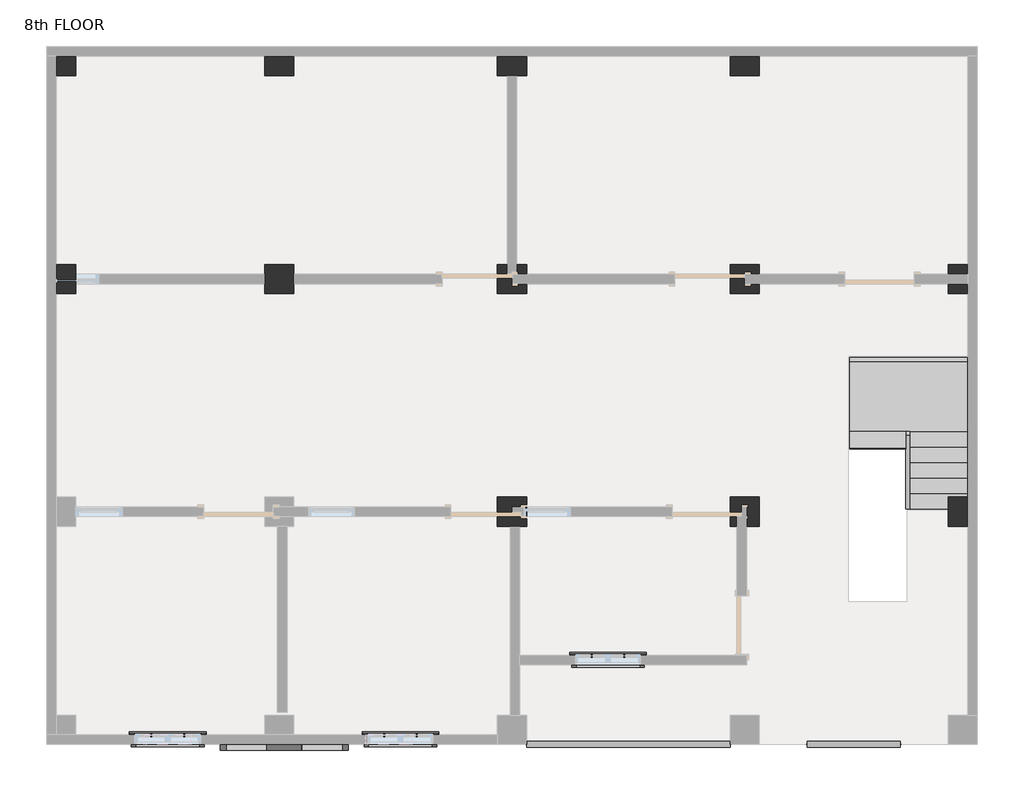
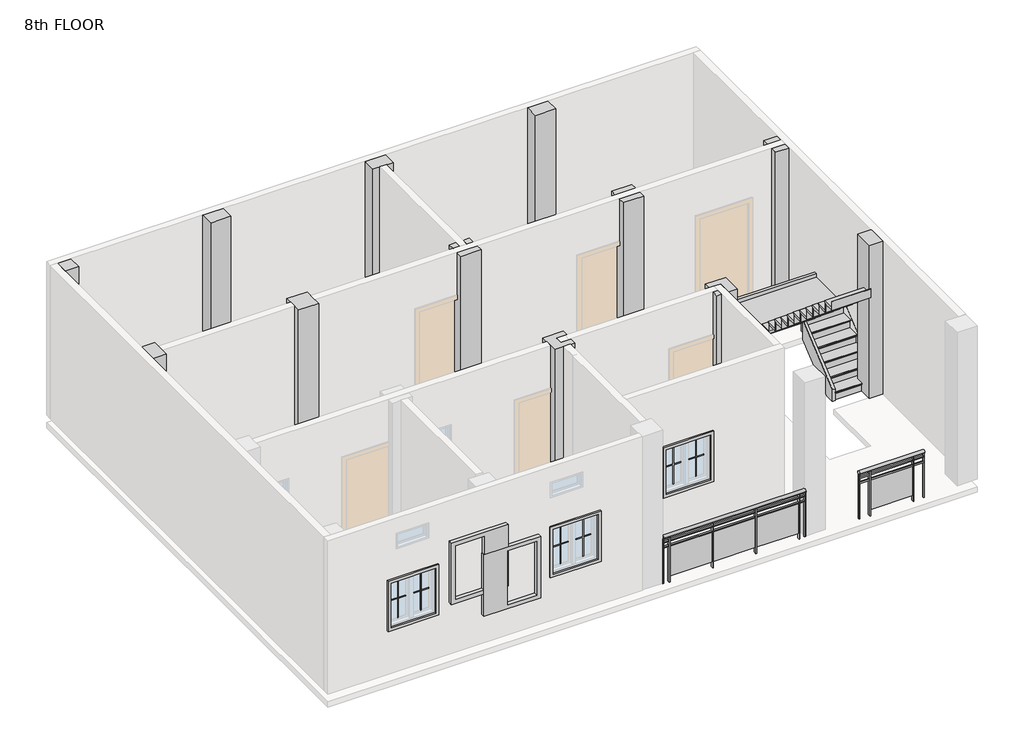
# One storey, part 2 of 2: 12 columns, 12 proxies, 4 members, 2 railings, 1 damper, 1 stair flight.
"""IFC4 building model written with IfcOpenShell, lengths in millimetres."""

from ifc_helpers import new_model, si_unit, point, frame, origin, place, context, project, spatial, polyline, ellipse_curve, trimmed, outline, extrude, faceted_brep, transform, mapped, element, save
from ifc_brep_helpers import plane_surface, extruded_surface, advanced_brep
from components import muntin_pattern_2x2_muntin_pattern_2x2_b3fe6957, muntin_pattern_2x2_muntin_pattern_2x2_3e0ecaf2, trim_window_exterior_flat_with_sill_41619996, trim_window_interior_flat_picture_frame_51c85655, duct_accessories_5_duct_accessories_1_bcda36b2, stair_flight_07a640bc

model = new_model("IFC4")

# Units and contexts
model_context = context("Model", 3, world=origin())
ifc_project = project(units=[si_unit("LENGTHUNIT", "METRE", prefix="MILLI")], contexts=[model_context])

# Site, building, storey
site = spatial("IfcSite", under=ifc_project)
building = spatial("IfcBuilding", under=site)
storey = spatial("IfcBuildingStorey", under=building, Name="8th FLOOR", Elevation=24231.6)

# Proxies
placement = place(None, origin())
muntin_pattern_2x2_muntin_pattern_2x2_shape = muntin_pattern_2x2_muntin_pattern_2x2_b3fe6957(model_context)
element("IfcBuildingElementProxy", 1, Name="Muntin Pattern_2x2 : Muntin Pattern_2x2", ObjectType="Muntin Pattern_2x2 : Muntin Pattern_2x2", at=placement, inside=storey, context=model_context, shape_type="MappedRepresentation", body=[
    mapped(muntin_pattern_2x2_muntin_pattern_2x2_shape, transform((-14441.409625, -253.8184478, 25215.85), x_axis=(1.0, 0.0, 0.0), y_axis=(0.0, 1.0, 0.0), z_axis=(0.0, 0.0, 1.0))),
])
element("IfcBuildingElementProxy", 2, Name="Muntin Pattern_2x2 : Muntin Pattern_2x2", ObjectType="Muntin Pattern_2x2 : Muntin Pattern_2x2", at=placement, inside=storey, context=model_context, shape_type="MappedRepresentation", body=[
    mapped(muntin_pattern_2x2_muntin_pattern_2x2_shape, transform((-11393.409625, -253.8184478, 25215.85), x_axis=(1.0, 0.0, 0.0), y_axis=(0.0, 1.0, 0.0), z_axis=(0.0, 0.0, 1.0))),
])
element("IfcBuildingElementProxy", 3, Name="Muntin Pattern_2x2 : Muntin Pattern_2x2", ObjectType="Muntin Pattern_2x2 : Muntin Pattern_2x2", at=placement, inside=storey, context=model_context, shape_type="MappedRepresentation", body=[
    mapped(muntin_pattern_2x2_muntin_pattern_2x2_shape, transform((-8675.609625, 787.5815522, 25215.85), x_axis=(1.0, 0.0, 0.0), y_axis=(0.0, 1.0, 0.0), z_axis=(0.0, 0.0, 1.0))),
])
muntin_pattern_2x2_muntin_pattern_2x2_2_shape = muntin_pattern_2x2_muntin_pattern_2x2_3e0ecaf2(model_context)
element("IfcBuildingElementProxy", 4, Name="Muntin Pattern_2x2 : Muntin Pattern_2x2", ObjectType="Muntin Pattern_2x2 : Muntin Pattern_2x2", at=placement, inside=storey, context=model_context, shape_type="MappedRepresentation", body=[
    mapped(muntin_pattern_2x2_muntin_pattern_2x2_2_shape, transform((-14012.784625, -253.8184478, 25215.85), x_axis=(-1.0, 0.0, 0.0), y_axis=(0.0, -1.0, 0.0), z_axis=(0.0, 0.0, 1.0))),
])
element("IfcBuildingElementProxy", 5, Name="Muntin Pattern_2x2 : Muntin Pattern_2x2", ObjectType="Muntin Pattern_2x2 : Muntin Pattern_2x2", at=placement, inside=storey, context=model_context, shape_type="MappedRepresentation", body=[
    mapped(muntin_pattern_2x2_muntin_pattern_2x2_2_shape, transform((-10964.784625, -253.8184478, 25215.85), x_axis=(-1.0, 0.0, 0.0), y_axis=(0.0, -1.0, 0.0), z_axis=(0.0, 0.0, 1.0))),
])
element("IfcBuildingElementProxy", 6, Name="Muntin Pattern_2x2 : Muntin Pattern_2x2", ObjectType="Muntin Pattern_2x2 : Muntin Pattern_2x2", at=placement, inside=storey, context=model_context, shape_type="MappedRepresentation", body=[
    mapped(muntin_pattern_2x2_muntin_pattern_2x2_2_shape, transform((-8246.984625, 787.5815522, 25215.85), x_axis=(-1.0, 0.0, 0.0), y_axis=(0.0, -1.0, 0.0), z_axis=(0.0, 0.0, 1.0))),
])
trim_window_exterior_flat_with_sill_shape = trim_window_exterior_flat_with_sill_41619996(model_context)
element("IfcBuildingElementProxy", 7, Name="Trim-Window-Exterior-Flat : with Sill", ObjectType="Trim-Window-Exterior-Flat : with Sill", at=placement, inside=storey, context=model_context, shape_type="MappedRepresentation", body=[
    mapped(trim_window_exterior_flat_with_sill_shape, transform((-14227.097125, -244.2934478, 26060.4), x_axis=(-1.0, 0.0, 0.0), y_axis=(0.0, 0.0, 1.0), z_axis=(0.0, 1.0, 0.0))),
])
element("IfcBuildingElementProxy", 8, Name="Trim-Window-Exterior-Flat : with Sill", ObjectType="Trim-Window-Exterior-Flat : with Sill", at=placement, inside=storey, context=model_context, shape_type="MappedRepresentation", body=[
    mapped(trim_window_exterior_flat_with_sill_shape, transform((-11179.097125, -244.2934478, 26060.4), x_axis=(-1.0, 0.0, 0.0), y_axis=(0.0, 0.0, 1.0), z_axis=(0.0, 1.0, 0.0))),
])
element("IfcBuildingElementProxy", 9, Name="Trim-Window-Exterior-Flat : with Sill", ObjectType="Trim-Window-Exterior-Flat : with Sill", at=placement, inside=storey, context=model_context, shape_type="MappedRepresentation", body=[
    mapped(trim_window_exterior_flat_with_sill_shape, transform((-8461.297125, 797.1065522, 26060.4), x_axis=(-1.0, 0.0, 0.0), y_axis=(0.0, 0.0, 1.0), z_axis=(0.0, 1.0, 0.0))),
])
trim_window_interior_flat_picture_frame_shape = trim_window_interior_flat_picture_frame_51c85655(model_context)
element("IfcBuildingElementProxy", 10, Name="Trim-Window-Interior-Flat : Picture Frame", ObjectType="Trim-Window-Interior-Flat : Picture Frame", at=placement, inside=storey, context=model_context, shape_type="MappedRepresentation", body=[
    mapped(trim_window_interior_flat_picture_frame_shape, transform((-14227.097125, -371.2934478, 26060.4), x_axis=(1.0, 0.0, 0.0), y_axis=(0.0, 0.0, 1.0), z_axis=(0.0, -1.0, 0.0))),
])
element("IfcBuildingElementProxy", 11, Name="Trim-Window-Interior-Flat : Picture Frame", ObjectType="Trim-Window-Interior-Flat : Picture Frame", at=placement, inside=storey, context=model_context, shape_type="MappedRepresentation", body=[
    mapped(trim_window_interior_flat_picture_frame_shape, transform((-11179.097125, -371.2934478, 26060.4), x_axis=(1.0, 0.0, 0.0), y_axis=(0.0, 0.0, 1.0), z_axis=(0.0, -1.0, 0.0))),
])
element("IfcBuildingElementProxy", 12, Name="Trim-Window-Interior-Flat : Picture Frame", ObjectType="Trim-Window-Interior-Flat : Picture Frame", at=placement, inside=storey, context=model_context, shape_type="MappedRepresentation", body=[
    mapped(trim_window_interior_flat_picture_frame_shape, transform((-8461.297125, 670.1065522, 26060.4), x_axis=(1.0, 0.0, 0.0), y_axis=(0.0, 0.0, 1.0), z_axis=(0.0, -1.0, 0.0))),
])

# Columns
element("IfcColumn", 13, ObjectType="column family : column family", at=placement, inside=storey, context=model_context, shape_type="SweptSolid", body=[
    extrude(outline(polyline([(-15433.597125, 8645.7065522), (-15433.597125, 8391.7065522), (-15687.597125, 8391.7065522), (-15687.597125, 8645.7065522), (-15433.597125, 8645.7065522)])), frame((0.0, 0.0, 24236.6), z_axis=(0.0, 0.0, 1.0), x_axis=(1.0, 0.0, 0.0)), (0.0, 0.0, 1.0), 3038.0),
])
element("IfcColumn", 14, ObjectType="column family : column family", at=placement, inside=storey, context=model_context, shape_type="SweptSolid", body=[
    extrude(outline(polyline([(-12576.097125, 5915.2065522), (-12576.097125, 5534.2065522), (-12957.097125, 5534.2065522), (-12957.097125, 5915.2065522), (-12576.097125, 5915.2065522)])), frame((0.0, 0.0, 24236.6), z_axis=(0.0, 0.0, 1.0), x_axis=(1.0, 0.0, 0.0)), (0.0, 0.0, 1.0), 3038.0),
])
element("IfcColumn", 15, ObjectType="column family : column family", at=placement, inside=storey, context=model_context, shape_type="Brep", body=[
    faceted_brep([(-9655.097125, 5915.2065522, 24236.6), (-9528.097125, 5915.2065522, 24236.6), (-9528.097125, 5788.2065522, 24236.6), (-9655.097125, 5788.2065522, 24236.6), (-9528.097125, 5915.2065522, 27274.6), (-9655.097125, 5915.2065522, 27274.6), (-9655.097125, 5788.2065522, 27274.6), (-9528.097125, 5788.2065522, 27274.6)], [[[0, 1, 2, 3]], [[4, 5, 6, 7]], [[0, 3, 6, 5]], [[4, 1, 0, 5]], [[3, 2, 7, 6]], [[1, 4, 7, 2]]]),
    faceted_brep([(-9528.097125, 5534.2065522, 27274.6), (-9528.097125, 5534.2065522, 24236.6), (-9528.097125, 5661.2065522, 24236.6), (-9528.097125, 5661.2065522, 27274.6), (-9909.097125, 5534.2065522, 24236.6), (-9909.097125, 5534.2065522, 27274.6), (-9909.097125, 5915.2065522, 24236.6), (-9909.097125, 5661.2065522, 27274.6), (-9909.097125, 5661.2065522, 26365.2), (-9909.097125, 5788.2065522, 26365.2), (-9909.097125, 5788.2065522, 27274.6), (-9909.097125, 5915.2065522, 27274.6), (-9782.097125, 5915.2065522, 27274.6), (-9782.097125, 5915.2065522, 24236.6), (-9782.097125, 5788.2065522, 24236.6), (-9782.097125, 5788.2065522, 27274.6), (-9782.097125, 5788.2065522, 26365.2), (-9718.597125, 5788.2065522, 24236.6), (-9718.597125, 5788.2065522, 26365.2), (-9718.597125, 5661.2065522, 24236.6), (-9718.597125, 5661.2065522, 26365.2)], [[[0, 1, 2, 3]], [[4, 1, 0, 5]], [[6, 4, 5, 7, 8, 9, 10, 11]], [[6, 11, 12, 13]], [[14, 13, 12, 15, 16]], [[17, 14, 16, 18]], [[19, 20, 8, 7, 3, 2]], [[1, 4, 6, 13, 14, 17, 19, 2]], [[5, 0, 3, 7]], [[12, 11, 10, 15]], [[9, 16, 15, 10]], [[18, 20, 19, 17]], [[20, 18, 16, 9, 8]]]),
])
element("IfcColumn", 16, ObjectType="column family : column family", at=placement, inside=storey, context=model_context, shape_type="Brep", body=[
    faceted_brep([(-6480.097125, 5534.2065522, 24236.6), (-6861.097125, 5534.2065522, 24236.6), (-6861.097125, 5915.2065522, 24236.6), (-6480.097125, 5915.2065522, 24236.6), (-6480.097125, 5788.2065522, 24236.6), (-6670.597125, 5788.2065522, 24236.6), (-6670.597125, 5661.2065522, 24236.6), (-6480.097125, 5661.2065522, 24236.6), (-6480.097125, 5534.2065522, 27274.6), (-6480.097125, 5661.2065522, 27274.6), (-6861.097125, 5534.2065522, 27274.6), (-6861.097125, 5661.2065522, 27274.6), (-6861.097125, 5661.2065522, 26365.2), (-6861.097125, 5788.2065522, 26365.2), (-6861.097125, 5788.2065522, 27274.6), (-6861.097125, 5915.2065522, 27274.6), (-6480.097125, 5915.2065522, 27274.6), (-6670.597125, 5661.2065522, 26365.2), (-6670.597125, 5788.2065522, 26365.2), (-6480.097125, 5788.2065522, 27274.6)], [[[0, 1, 2, 3, 4, 5, 6, 7]], [[8, 0, 7, 9]], [[1, 0, 8, 10]], [[2, 1, 10, 11, 12, 13, 14, 15]], [[3, 2, 15, 16]], [[10, 8, 9, 11]], [[6, 17, 12, 11, 9, 7]], [[13, 18, 5, 4, 19, 14]], [[3, 16, 19, 4]], [[16, 15, 14, 19]], [[18, 17, 6, 5]], [[17, 18, 13, 12]]]),
])
element("IfcColumn", 17, ObjectType="column family : column family", at=placement, inside=storey, context=model_context, shape_type="Brep", body=[
    faceted_brep([(-6480.097125, 2867.2065522, 24236.6), (-6480.097125, 2486.2065522, 24236.6), (-6645.197125, 2486.2065522, 24236.6), (-6645.197125, 2740.2065522, 24236.6), (-6708.697125, 2740.2065522, 24236.6), (-6708.697125, 2613.2065522, 24236.6), (-6772.197125, 2613.2065522, 24236.6), (-6772.197125, 2486.2065522, 24236.6), (-6861.097125, 2486.2065522, 24236.6), (-6861.097125, 2867.2065522, 24236.6), (-6480.097125, 2867.2065522, 27274.6), (-6480.097125, 2486.2065522, 27274.6), (-6861.097125, 2486.2065522, 27274.6), (-6772.197125, 2486.2065522, 27274.6), (-6861.097125, 2613.2065522, 27274.6), (-6861.097125, 2613.2065522, 26365.2), (-6861.097125, 2740.2065522, 26365.2), (-6861.097125, 2740.2065522, 27274.6), (-6861.097125, 2867.2065522, 27274.6), (-6772.197125, 2740.2065522, 27274.6), (-6645.197125, 2740.2065522, 27274.6), (-6645.197125, 2486.2065522, 27274.6), (-6772.197125, 2613.2065522, 27274.6), (-6772.197125, 2613.2065522, 26365.2), (-6772.197125, 2740.2065522, 26365.2), (-6708.697125, 2613.2065522, 26365.2), (-6708.697125, 2740.2065522, 26365.2)], [[[0, 1, 2, 3, 4, 5, 6, 7, 8, 9]], [[1, 0, 10, 11]], [[12, 8, 7, 13]], [[9, 8, 12, 14, 15, 16, 17, 18]], [[0, 9, 18, 10]], [[11, 10, 18, 17, 19, 20, 21]], [[15, 14, 22, 23]], [[17, 16, 24, 19]], [[20, 3, 2, 21]], [[6, 23, 22, 13, 7]], [[14, 12, 13, 22]], [[1, 11, 21, 2]], [[15, 23, 24, 16]], [[25, 23, 6, 5]], [[23, 25, 26, 24]], [[26, 25, 5, 4]], [[24, 26, 4, 3, 20, 19]]]),
])
element("IfcColumn", 18, ObjectType="column family : column family", at=placement, inside=storey, context=model_context, shape_type="Brep", body=[
    faceted_brep([(-9528.097125, 2486.2065522, 24236.6), (-9909.097125, 2486.2065522, 24236.6), (-9909.097125, 2867.2065522, 24236.6), (-9528.097125, 2867.2065522, 24236.6), (-9528.097125, 2740.2065522, 24236.6), (-9566.197125, 2740.2065522, 24236.6), (-9718.597125, 2740.2065522, 24236.6), (-9718.597125, 2613.2065522, 24236.6), (-9566.197125, 2613.2065522, 24236.6), (-9528.097125, 2613.2065522, 24236.6), (-9528.097125, 2486.2065522, 27274.6), (-9528.097125, 2613.2065522, 24536.4), (-9528.097125, 2740.2065522, 24536.4), (-9528.097125, 2867.2065522, 27274.6), (-9528.097125, 2740.2065522, 27274.6), (-9528.097125, 2740.2065522, 26365.2), (-9528.097125, 2613.2065522, 26365.2), (-9528.097125, 2613.2065522, 27274.6), (-9909.097125, 2486.2065522, 27274.6), (-9909.097125, 2867.2065522, 27274.6), (-9566.197125, 2613.2065522, 27274.6), (-9718.597125, 2613.2065522, 27274.6), (-9718.597125, 2740.2065522, 27274.6), (-9566.197125, 2740.2065522, 27274.6), (-9566.197125, 2613.2065522, 26365.2), (-9566.197125, 2613.2065522, 24536.4), (-9566.197125, 2740.2065522, 24536.4), (-9566.197125, 2740.2065522, 26365.2)], [[[0, 1, 2, 3, 4, 5, 6, 7, 8, 9]], [[10, 0, 9, 11, 12, 4, 3, 13, 14, 15, 16, 17]], [[1, 0, 10, 18]], [[2, 1, 18, 19]], [[3, 2, 19, 13]], [[18, 10, 17, 20, 21, 22, 23, 14, 13, 19]], [[11, 9, 8, 7, 21, 20, 17, 16, 24, 25]], [[4, 12, 26, 27, 15, 14, 23, 22, 6, 5]], [[21, 7, 6, 22]], [[25, 24, 27, 26]], [[25, 26, 12, 11]], [[27, 24, 16, 15]]]),
])
element("IfcColumn", 19, ObjectType="column family : column family", at=placement, inside=storey, context=model_context, shape_type="SweptSolid", body=[
    extrude(outline(polyline([(-12576.097125, 8391.7065522), (-12957.097125, 8391.7065522), (-12957.097125, 8645.7065522), (-12576.097125, 8645.7065522), (-12576.097125, 8391.7065522)])), frame((0.0, 0.0, 24236.6), z_axis=(0.0, 0.0, 1.0), x_axis=(1.0, 0.0, 0.0)), (0.0, 0.0, 1.0), 3038.0),
])
element("IfcColumn", 20, ObjectType="column family : column family", at=placement, inside=storey, context=model_context, shape_type="SweptSolid", body=[
    extrude(outline(polyline([(-9528.097125, 8391.7065522), (-9909.097125, 8391.7065522), (-9909.097125, 8645.7065522), (-9528.097125, 8645.7065522), (-9528.097125, 8391.7065522)])), frame((0.0, 0.0, 24236.6), z_axis=(0.0, 0.0, 1.0), x_axis=(1.0, 0.0, 0.0)), (0.0, 0.0, 1.0), 3038.0),
])
element("IfcColumn", 21, ObjectType="column family : column family", at=placement, inside=storey, context=model_context, shape_type="SweptSolid", body=[
    extrude(outline(polyline([(-6480.097125, 8391.7065522), (-6861.097125, 8391.7065522), (-6861.097125, 8645.7065522), (-6480.097125, 8645.7065522), (-6480.097125, 8391.7065522)])), frame((0.0, 0.0, 24236.6), z_axis=(0.0, 0.0, 1.0), x_axis=(1.0, 0.0, 0.0)), (0.0, 0.0, 1.0), 3038.0),
])
element("IfcColumn", 22, ObjectType="column family : column family", at=placement, inside=storey, context=model_context, shape_type="SweptSolid", body=[
    extrude(outline(polyline([(-4003.597125, 5915.2065522), (-3749.597125, 5915.2065522), (-3749.597125, 5788.2065522), (-4003.597125, 5788.2065522), (-4003.597125, 5915.2065522)])), frame((0.0, 0.0, 24236.6), z_axis=(0.0, 0.0, 1.0), x_axis=(1.0, 0.0, 0.0)), (0.0, 0.0, 1.0), 3038.0),
    extrude(outline(polyline([(-3749.597125, 5534.2065522), (-4003.597125, 5534.2065522), (-4003.597125, 5661.2065522), (-3749.597125, 5661.2065522), (-3749.597125, 5534.2065522)])), frame((0.0, 0.0, 24236.6), z_axis=(0.0, 0.0, 1.0), x_axis=(1.0, 0.0, 0.0)), (0.0, 0.0, 1.0), 3038.0),
])
element("IfcColumn", 23, ObjectType="column family : column family", at=placement, inside=storey, context=model_context, shape_type="SweptSolid", body=[
    extrude(outline(polyline([(-4003.597125, 2486.2065522), (-4003.597125, 2867.2065522), (-3749.597125, 2867.2065522), (-3749.597125, 2486.2065522), (-4003.597125, 2486.2065522)])), frame((0.0, 0.0, 24236.6), z_axis=(0.0, 0.0, 1.0), x_axis=(1.0, 0.0, 0.0)), (0.0, 0.0, 1.0), 3038.0),
])
element("IfcColumn", 24, ObjectType="column family : column family", at=placement, inside=storey, context=model_context, shape_type="SweptSolid", body=[
    extrude(outline(polyline([(-15433.597125, 5915.2065522), (-15433.597125, 5534.2065522), (-15687.597125, 5534.2065522), (-15687.597125, 5915.2065522), (-15433.597125, 5915.2065522)])), frame((0.0, 0.0, 24236.6), z_axis=(0.0, 0.0, 1.0), x_axis=(1.0, 0.0, 0.0)), (0.0, 0.0, 1.0), 3038.0),
])

# Damper
duct_accessories_5_duct_accessories_1_shape = duct_accessories_5_duct_accessories_1_bcda36b2(model_context)
element("IfcDamper", 25, ObjectType="Duct Accessories 5 : Duct Accessories 1", at=placement, inside=storey, context=model_context, shape_type="MappedRepresentation", body=[
    mapped(duct_accessories_5_duct_accessories_1_shape, transform((0.0, 0.0, 0.0), x_axis=(1.0, 0.0, 0.0), y_axis=(0.0, 1.0, 0.0), z_axis=(0.0, 0.0, 1.0))),
])

# Members
element("IfcMember", 26, ObjectType="Stringer - 2\" Width", at=placement, inside=storey, context=model_context, shape_type="SweptSolid", body=[
    extrude(outline(polyline([(2714.6319226, 24231.6), (2714.6319226, 24468.4438745), (3679.8319226, 25272.7772078), (3679.8319226, 24876.0165243), (2906.5320935, 24231.6), (2714.6319226, 24231.6)])), frame((-4563.0136682, 0.0, 0.0), z_axis=(1.0, 0.0, 0.0), x_axis=(0.0, 1.0, 0.0)), (0.0, 0.0, 1.0), 50.8),
])
element("IfcMember", 27, ObjectType="Stringer - 2\" Width", at=placement, inside=storey, context=model_context, shape_type="SweptSolid", body=[
    extrude(outline(polyline([(-4512.2136682, 3730.6319226), (-4512.2136682, 3679.8319226), (-4563.0136682, 3679.8319226), (-4563.0136682, 3730.6319226), (-4512.2136682, 3730.6319226)])), frame((0.0, 0.0, 25019.0), z_axis=(0.0, 0.0, 1.0), x_axis=(1.0, 0.0, 0.0)), (0.0, 0.0, 1.0), 304.8),
])
element("IfcMember", 28, ObjectType="Stringer - 2\" Width", at=placement, inside=storey, context=model_context, shape_type="SweptSolid", body=[
    extrude(outline(polyline([(2714.6319226, 24231.6), (2714.6319226, 24468.4438745), (3741.0592732, 25323.8), (4217.1720935, 25323.8), (2906.5320935, 24231.6), (2714.6319226, 24231.6)])), frame((-3749.597125, 0.0, 0.0), z_axis=(1.0, 0.0, 0.0), x_axis=(0.0, 1.0, 0.0)), (0.0, 0.0, 1.0), 50.8),
])
element("IfcMember", 29, ObjectType="Stringer - 2\" Width", at=placement, inside=storey, context=model_context, shape_type="SweptSolid", body=[
    extrude(outline(polyline([(-3698.797125, 4695.8319226), (-3698.797125, 4645.0319226), (-5295.0246464, 4645.0319226), (-5295.0246464, 4695.8319226), (-3698.797125, 4695.8319226)])), frame((0.0, 0.0, 25019.0), z_axis=(0.0, 0.0, 1.0), x_axis=(1.0, 0.0, 0.0)), (0.0, 0.0, 1.0), 304.8),
])

# Railings
element("IfcRailing", 30, ObjectType="Glass Panel - Bottom Fill", at=placement, inside=storey, context=model_context, shape_type="SolidModel", body=[
    advanced_brep(
    [(-9528.097125, -333.1934478, 25146.0), (-9528.097125, -409.3934478, 25146.0), (-6861.097125, -333.1934478, 25146.0), (-6861.097125, -409.3934478, 25146.0)],
    [
        (0, 1, ellipse_curve(frame((-9528.097125, -371.2934478, 25146.0), z_axis=(-1.0, 0.0, 0.0), x_axis=(0.0, -1.0, 0.0)), 38.1, 28.575)),
        (1, 0, ellipse_curve(frame((-9528.097125, -371.2934478, 25146.0), z_axis=(-1.0, 0.0, 0.0), x_axis=(0.0, -1.0, 0.0)), 38.1, 28.575)),
        (2, 3, ellipse_curve(frame((-6861.097125, -371.2934478, 25146.0), z_axis=(1.0, 0.0, 0.0), x_axis=(0.0, -1.0, 0.0)), 38.1, 28.575)),
        (3, 2, ellipse_curve(frame((-6861.097125, -371.2934478, 25146.0), z_axis=(1.0, 0.0, 0.0), x_axis=(0.0, -1.0, 0.0)), 38.1, 28.575)),
        (0, 2),
        (3, 1),
    ],
    [
        plane_surface(frame((-9528.097125, -371.2934478, 25146.0), z_axis=(-1.0, 0.0, 0.0), x_axis=(0.0, 1.0, 0.0))),
        plane_surface(frame((-6861.097125, -371.2934478, 25146.0), z_axis=(1.0, 0.0, 0.0), x_axis=(0.0, 1.0, 0.0))),
        extruded_surface(trimmed(ellipse_curve(frame((-6861.097125, -371.2934478, 25146.0), z_axis=(-1.0, 0.0, 0.0), x_axis=(0.0, -1.0, 0.0)), 38.1, 28.575), [point((-6861.097125, -333.1934478, 25146.0))], [point((-6861.097125, -409.3934478, 25146.0))], True, "CARTESIAN"), (-2667.0, 0.0, 0.0), 2667.0),
        extruded_surface(trimmed(ellipse_curve(frame((-6861.097125, -371.2934478, 25146.0), z_axis=(-1.0, 0.0, 0.0), x_axis=(0.0, -1.0, 0.0)), 38.1, 28.575), [point((-6861.097125, -409.3934478, 25146.0))], [point((-6861.097125, -333.1934478, 25146.0))], True, "CARTESIAN"), (-2667.0, 0.0, 0.0), 2667.0),
    ],
    [
        (0, [[1, 2]]),
        (1, [[3, 4]]),
        (2, [[-1, 5, -4, 6]]),
        (3, [[-2, -6, -3, -5]]),
    ],
),
    extrude(outline(polyline([(-9528.097125, -383.9934478), (-9528.097125, -358.5934478), (-6861.097125, -358.5934478), (-6861.097125, -383.9934478), (-9528.097125, -383.9934478)])), frame((0.0, 0.0, 25031.7), z_axis=(0.0, 0.0, 1.0), x_axis=(1.0, 0.0, 0.0)), (0.0, 0.0, 1.0), 25.4),
    extrude(outline(polyline([(-9528.097125, -383.9934478), (-9528.097125, -358.5934478), (-6861.097125, -358.5934478), (-6861.097125, -383.9934478), (-9528.097125, -383.9934478)])), frame((0.0, 0.0, 24930.1), z_axis=(0.0, 0.0, 1.0), x_axis=(1.0, 0.0, 0.0)), (0.0, 0.0, 1.0), 25.4),
    extrude(outline(polyline([(-6981.747125, -396.6934478), (-6981.747125, -345.8934478), (-6969.047125, -345.8934478), (-6969.047125, -396.6934478), (-6981.747125, -396.6934478)])), frame((0.0, 0.0, 24231.6), z_axis=(0.0, 0.0, 1.0), x_axis=(1.0, 0.0, 0.0)), (0.0, 0.0, 1.0), 885.6788223),
    extrude(outline(polyline([(-7788.197125, -364.7582908), (-6975.397125, -364.7582908), (-6975.397125, -371.1082908), (-7788.197125, -371.1082908), (-7788.197125, -364.7582908)])), frame((0.0, 0.0, 24333.2), z_axis=(0.0, 0.0, 1.0), x_axis=(1.0, 0.0, 0.0)), (0.0, 0.0, 1.0), 596.9),
    extrude(outline(polyline([(-7794.547125, -396.6934478), (-7794.547125, -345.8934478), (-7781.847125, -345.8934478), (-7781.847125, -396.6934478), (-7794.547125, -396.6934478)])), frame((0.0, 0.0, 24231.6), z_axis=(0.0, 0.0, 1.0), x_axis=(1.0, 0.0, 0.0)), (0.0, 0.0, 1.0), 885.6788223),
    extrude(outline(polyline([(-8600.997125, -364.7582908), (-7788.197125, -364.7582908), (-7788.197125, -371.1082908), (-8600.997125, -371.1082908), (-8600.997125, -364.7582908)])), frame((0.0, 0.0, 24333.2), z_axis=(0.0, 0.0, 1.0), x_axis=(1.0, 0.0, 0.0)), (0.0, 0.0, 1.0), 596.9),
    extrude(outline(polyline([(-8607.347125, -396.6934478), (-8607.347125, -345.8934478), (-8594.647125, -345.8934478), (-8594.647125, -396.6934478), (-8607.347125, -396.6934478)])), frame((0.0, 0.0, 24231.6), z_axis=(0.0, 0.0, 1.0), x_axis=(1.0, 0.0, 0.0)), (0.0, 0.0, 1.0), 885.6788223),
    extrude(outline(polyline([(-9413.797125, -364.7582908), (-8600.997125, -364.7582908), (-8600.997125, -371.1082908), (-9413.797125, -371.1082908), (-9413.797125, -364.7582908)])), frame((0.0, 0.0, 24333.2), z_axis=(0.0, 0.0, 1.0), x_axis=(1.0, 0.0, 0.0)), (0.0, 0.0, 1.0), 596.9),
    extrude(outline(polyline([(-9420.147125, -396.6934478), (-9420.147125, -345.8934478), (-9407.447125, -345.8934478), (-9407.447125, -396.6934478), (-9420.147125, -396.6934478)])), frame((0.0, 0.0, 24231.6), z_axis=(0.0, 0.0, 1.0), x_axis=(1.0, 0.0, 0.0)), (0.0, 0.0, 1.0), 885.6788223),
    extrude(outline(polyline([(-6873.797125, -380.8184478), (-6873.797125, -361.7684478), (-6854.747125, -361.7684478), (-6854.747125, -380.8184478), (-6873.797125, -380.8184478)])), frame((0.0, 0.0, 24231.6), z_axis=(0.0, 0.0, 1.0), x_axis=(1.0, 0.0, 0.0)), (0.0, 0.0, 1.0), 885.6788223),
    extrude(outline(polyline([(-9534.447125, -380.8184478), (-9534.447125, -361.7684478), (-9515.397125, -361.7684478), (-9515.397125, -380.8184478), (-9534.447125, -380.8184478)])), frame((0.0, 0.0, 24231.6), z_axis=(0.0, 0.0, 1.0), x_axis=(1.0, 0.0, 0.0)), (0.0, 0.0, 1.0), 885.6788223),
])
element("IfcRailing", 31, ObjectType="Glass Panel - Bottom Fill", at=placement, inside=storey, context=model_context, shape_type="SolidModel", body=[
    advanced_brep(
    [(-5851.447125, -333.1934478, 25146.0), (-5851.447125, -409.3934478, 25146.0), (-4632.247125, -333.1934478, 25146.0), (-4632.247125, -409.3934478, 25146.0)],
    [
        (0, 1, ellipse_curve(frame((-5851.447125, -371.2934478, 25146.0), z_axis=(-1.0, 0.0, 0.0), x_axis=(0.0, -1.0, 0.0)), 38.1, 28.575)),
        (1, 0, ellipse_curve(frame((-5851.447125, -371.2934478, 25146.0), z_axis=(-1.0, 0.0, 0.0), x_axis=(0.0, -1.0, 0.0)), 38.1, 28.575)),
        (2, 3, ellipse_curve(frame((-4632.247125, -371.2934478, 25146.0), z_axis=(1.0, 0.0, 0.0), x_axis=(0.0, -1.0, 0.0)), 38.1, 28.575)),
        (3, 2, ellipse_curve(frame((-4632.247125, -371.2934478, 25146.0), z_axis=(1.0, 0.0, 0.0), x_axis=(0.0, -1.0, 0.0)), 38.1, 28.575)),
        (0, 2),
        (3, 1),
    ],
    [
        plane_surface(frame((-5851.447125, -371.2934478, 25146.0), z_axis=(-1.0, 0.0, 0.0), x_axis=(0.0, 1.0, 0.0))),
        plane_surface(frame((-4632.247125, -371.2934478, 25146.0), z_axis=(1.0, 0.0, 0.0), x_axis=(0.0, 1.0, 0.0))),
        extruded_surface(trimmed(ellipse_curve(frame((-4632.247125, -371.2934478, 25146.0), z_axis=(-1.0, 0.0, 0.0), x_axis=(0.0, -1.0, 0.0)), 38.1, 28.575), [point((-4632.247125, -333.1934478, 25146.0))], [point((-4632.247125, -409.3934478, 25146.0))], True, "CARTESIAN"), (-1219.1999999999998, 0.0, 0.0), 1219.1999999999998),
        extruded_surface(trimmed(ellipse_curve(frame((-4632.247125, -371.2934478, 25146.0), z_axis=(-1.0, 0.0, 0.0), x_axis=(0.0, -1.0, 0.0)), 38.1, 28.575), [point((-4632.247125, -409.3934478, 25146.0))], [point((-4632.247125, -333.1934478, 25146.0))], True, "CARTESIAN"), (-1219.1999999999998, 0.0, 0.0), 1219.1999999999998),
    ],
    [
        (0, [[1, 2]]),
        (1, [[3, 4]]),
        (2, [[-1, 5, -4, 6]]),
        (3, [[-2, -6, -3, -5]]),
    ],
),
    extrude(outline(polyline([(-5851.447125, -383.9934478), (-5851.447125, -358.5934478), (-4632.247125, -358.5934478), (-4632.247125, -383.9934478), (-5851.447125, -383.9934478)])), frame((0.0, 0.0, 25031.7), z_axis=(0.0, 0.0, 1.0), x_axis=(1.0, 0.0, 0.0)), (0.0, 0.0, 1.0), 25.4),
    extrude(outline(polyline([(-5851.447125, -383.9934478), (-5851.447125, -358.5934478), (-4632.247125, -358.5934478), (-4632.247125, -383.9934478), (-5851.447125, -383.9934478)])), frame((0.0, 0.0, 24930.1), z_axis=(0.0, 0.0, 1.0), x_axis=(1.0, 0.0, 0.0)), (0.0, 0.0, 1.0), 25.4),
    extrude(outline(polyline([(-4841.797125, -396.6934478), (-4841.797125, -345.8934478), (-4829.097125, -345.8934478), (-4829.097125, -396.6934478), (-4841.797125, -396.6934478)])), frame((0.0, 0.0, 24231.6), z_axis=(0.0, 0.0, 1.0), x_axis=(1.0, 0.0, 0.0)), (0.0, 0.0, 1.0), 885.6788223),
    extrude(outline(polyline([(-5648.247125, -364.7582908), (-4835.447125, -364.7582908), (-4835.447125, -371.1082908), (-5648.247125, -371.1082908), (-5648.247125, -364.7582908)])), frame((0.0, 0.0, 24333.2), z_axis=(0.0, 0.0, 1.0), x_axis=(1.0, 0.0, 0.0)), (0.0, 0.0, 1.0), 596.9),
    extrude(outline(polyline([(-5654.597125, -396.6934478), (-5654.597125, -345.8934478), (-5641.897125, -345.8934478), (-5641.897125, -396.6934478), (-5654.597125, -396.6934478)])), frame((0.0, 0.0, 24231.6), z_axis=(0.0, 0.0, 1.0), x_axis=(1.0, 0.0, 0.0)), (0.0, 0.0, 1.0), 885.6788223),
    extrude(outline(polyline([(-4644.947125, -380.8184478), (-4644.947125, -361.7684478), (-4625.897125, -361.7684478), (-4625.897125, -380.8184478), (-4644.947125, -380.8184478)])), frame((0.0, 0.0, 24231.6), z_axis=(0.0, 0.0, 1.0), x_axis=(1.0, 0.0, 0.0)), (0.0, 0.0, 1.0), 885.6788223),
    extrude(outline(polyline([(-5857.797125, -380.8184478), (-5857.797125, -361.7684478), (-5838.747125, -361.7684478), (-5838.747125, -380.8184478), (-5857.797125, -380.8184478)])), frame((0.0, 0.0, 24231.6), z_axis=(0.0, 0.0, 1.0), x_axis=(1.0, 0.0, 0.0)), (0.0, 0.0, 1.0), 885.6788223),
])

# Stair flight
stair_flight_shape = stair_flight_07a640bc(model_context)
element("IfcStairFlight", 32, ObjectType="2\" Tread 1\" Nosing 1/4\" Riser", at=placement, inside=storey, context=model_context, shape_type="MappedRepresentation", body=[
    mapped(stair_flight_shape, transform((0.0, 0.0, 0.0), x_axis=(1.0, 0.0, 0.0), y_axis=(0.0, 1.0, 0.0), z_axis=(0.0, 0.0, 1.0))),
])

save(model, "model.ifc")

# Revit data of these elements
# Type "Muntin Pattern_2x2 : Muntin Pattern_2x2"
#   Width [instance default] = 4' - 0"
#   Thickness = 0' - 0 1/2"
#   Height [instance default] = 4' - 0"
#   Distance = 0' - 0 3/4"
#   Interior Material [instance default] = none
#   Exterior Material [instance default] = none
#   Default Elevation = 0
# Type "Trim-Window-Exterior-Flat : with Sill"
#   Trim Width = 0' - 2 1/4"
#   Trim Thickness_Picture Frame = 0' - 1 1/4"
#   Trim Thickness_with Sill = 0' - 0 3/4"
#   Sill Thickness = 0' - 1 1/4"
#   Opening Width [instance default] = 2' - 0"
#   Opening Height [instance default] = 3' - 0"
#   Default Elevation = 4' - 0"
#   Sill = yes
#   Picture Frame = no
#   Trim Material [instance default] = none
# Type "Trim-Window-Interior-Flat : Picture Frame"
#   Trim Thickness_Picture Frame = 0' - 1 1/4"
#   Trim Width = 0' - 2 1/4"
#   Trim Thickness_with Sill = 0' - 0 3/4"
#   Sill Thickness = 0' - 1 1/4"
#   Opening Width [instance default] = 2' - 0"
#   Opening Height [instance default] = 3' - 0"
#   Default Elevation = 4' - 0"
#   Sill = no
#   Picture Frame = yes
#   Trim Material [instance default] = none
# Type "column family : column family"
#   w2 [instance default] = 0' - 9.88189"
#   w1 [instance default] = 0' - 9.01575"
#   Depth = 1' - 11.62205"
#   Width = 1' - 11.62205"
# Type "Glass Panel - Bottom Fill"
#   Assembly Code = "C2010400"
#   built-in parameter 1008612 = 0.0416667 (stored number, unit not read)
#   built-in parameter 1008611 = 0.0416667 (stored number, unit not read)
#   built-in parameter 1008609 = 0.333333 (stored number, unit not read)
#   built-in parameter 1008604 = 0.166667 (stored number, unit not read)
#   built-in parameter 1008603 = 0.166667 (stored number, unit not read)
#   Railing Height = 3' - 0"
#   built-in parameter 1008630 = 2
#   built-in parameter 1008610 = 2
#   built-in parameter 1008618 = Baluster - Square : 3/4"
# Elements 1, 2, 3, 4, 5, 6 (IfcBuildingElementProxy, "Muntin Pattern_2x2 : Muntin Pattern_2x2")
#   Width = 0' - 11 5/8"
#   Height = 2' - 6 1/2"
#   Interior Material = Wood - Stained
#   Exterior Material = Clad - White
#   Phase Created = New Construction
#   Materials on its faces: "Clad - White", "Wood - Stained"
# Elements 7, 8, 9 (IfcBuildingElementProxy, "Trim-Window-Exterior-Flat : with Sill")
#   Opening Width = 2' - 10"
#   Opening Height = 3' - 0"
#   Trim Material = Clad - White
#   Phase Created = New Construction
#   Materials on its faces: "Clad - White"
# Elements 10, 11, 12 (IfcBuildingElementProxy, "Trim-Window-Interior-Flat : Picture Frame")
#   Opening Width = 2' - 10"
#   Opening Height = 3' - 0"
#   Trim Material = Wood - Stained
#   Phase Created = New Construction
#   Materials on its faces: "Wood - Stained"
# Elements 13, 14, 15, 19, 20, 21 (IfcColumn, "column family : column family")
#   w2 = 1' - 3"
#   w1 = 1' - 3"
#   Phase Created = New Construction
#   Materials on its faces: "Default Wall"
# Elements 16, 22, 23 (IfcColumn, "column family : column family")
#   w2 = 1' - 3"
#   w1 = 1' - 3"
#   Phase Created = New Construction
#   Materials on its faces: "grey", "Default Wall"
# Elements 17, 18 (IfcColumn, "column family : column family")
#   w2 = 1' - 3"
#   w1 = 1' - 3"
#   Phase Created = New Construction
#   Materials on its faces: "Default Wall", "inside wall"
# Element 24 (IfcColumn, "column family : column family")
#   w2 = 1' - 3"
#   w1 = 1' - 3"
#   Phase Created = New Construction
#   Materials on its faces: "inside wall", "Default Wall"
# Element 25 (IfcDamper, "Duct Accessories 5 : Duct Accessories 1")
#   Mark = "5"
#   Phase Created = New Construction
#   Materials on its faces: "border"
# Elements 26, 27, 28, 29 (IfcMember, "Stringer - 2\" Width")
#   Phase Created = New Construction
# Elements 30, 31 (IfcRailing, "Glass Panel - Bottom Fill")
#   Phase Created = New Construction
#   Materials on its faces: "Glass"
# Element 32 (IfcStairFlight, "2\" Tread 1\" Nosing 1/4\" Riser")
#   Phase Created = New Construction
# Materials
#   "Clad - White": class "Wood", colour RGB 242 242 238, transparency 0, Cost = 0
#   "Wood - Stained": class "Wood", colour RGB 224 178 126, transparency 0, Cost = 0
#   "Default Wall": colour RGB 128 128 128, transparency 0, Cost = 0
#   "grey": class "Generic", colour RGB 80 80 80, transparency 0, Cost = 0
#   "inside wall": class "Generic", colour RGB 199 224 95, transparency 0, Cost = 0
#   "border": class "Generic", colour RGB 144 144 144, transparency 0, Cost = 0
#   "Glass": class "Glass", colour RGB 0 128 192, transparency 0.75, Description = "Soda Lime Glass", Cost = 0
